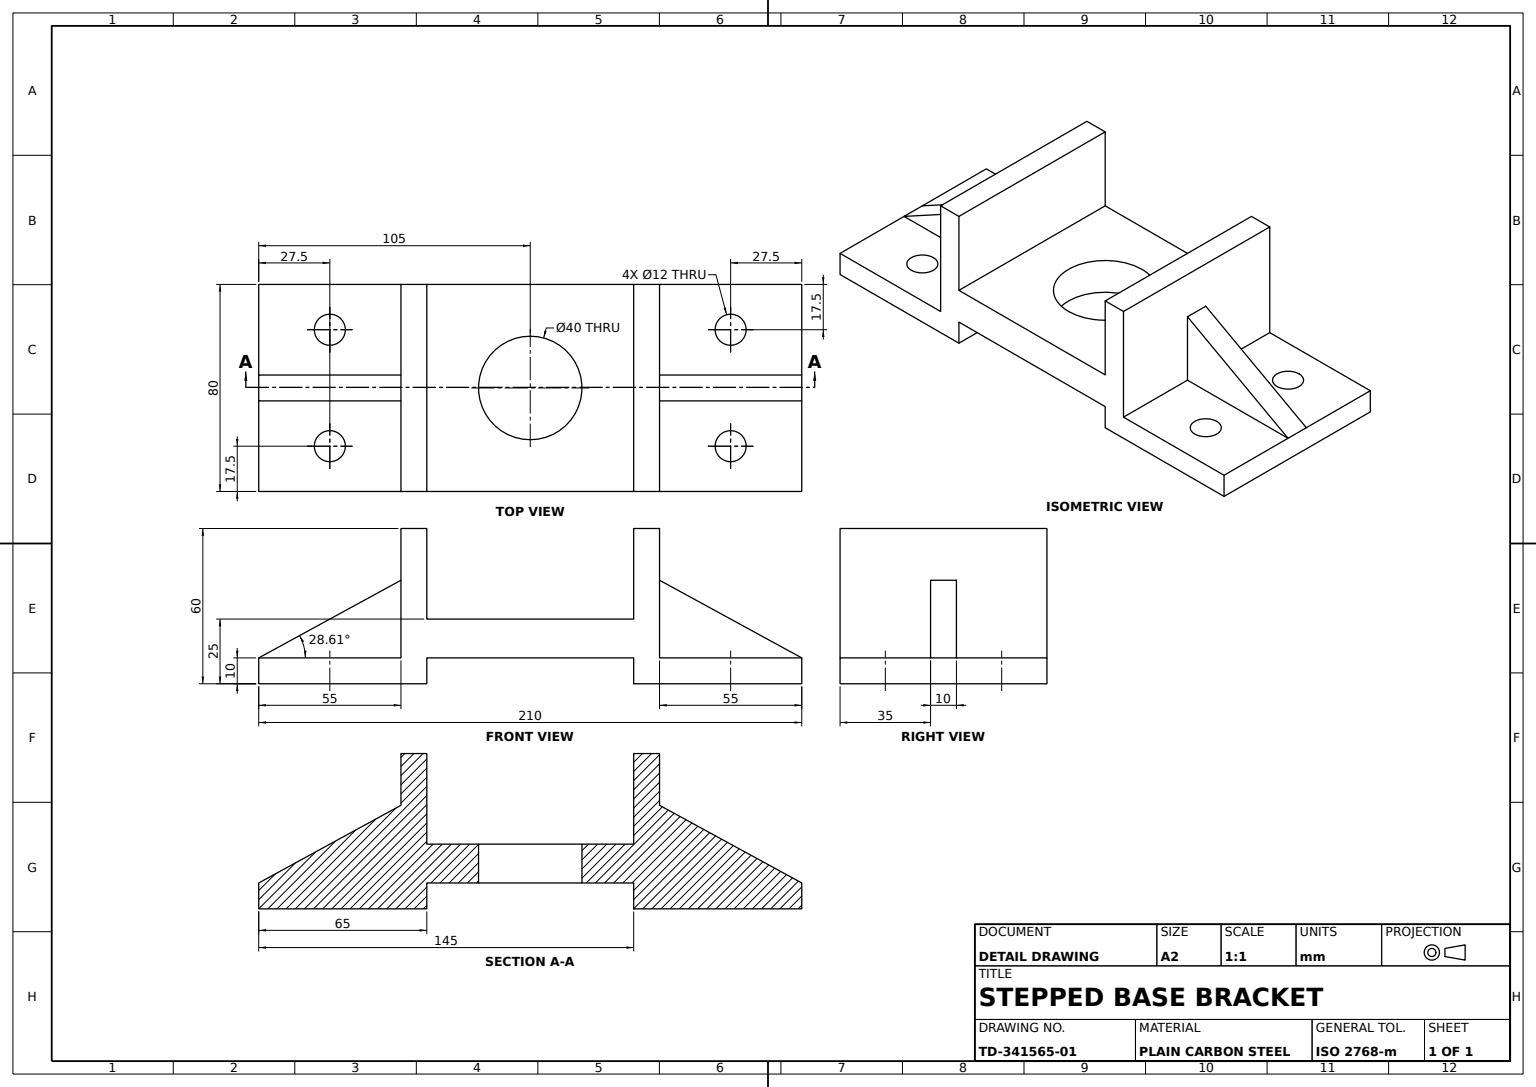
from build123d import *

# Parameters (mm, degrees)
BASE_BODY_DEPTH          = 60
CENTER_BORE_SKETCH_R     = 20
CENTER_BORE_DEPTH        = 15
GUSSET_1_BLANK_DEPTH     = 40
GUSSET_1_TRIM_A_DEPTH    = 25
GUSSET_1_TRIM_B_DEPTH    = 5
GUSSET_2_BLANK_DEPTH     = 35
GUSSET_2_TRIM_DEPTH      = 25
FLANGE_EXTENSION_1_DEPTH = 10
FLANGE_EXTENSION_2_DEPTH = 10
MOUNTING_HOLES_SKETCH_R  = 6
MOUNTING_HOLES_4X_DEPTH  = 10


with BuildPart() as part:
    # Base Profile Sketch → Base Body (new body)
    with BuildSketch(Plane.XY):
        Polygon((0, 0), (55, 0), (65, 0), (65, 10), (145, 10), (145, 0), (210, 0), (210, 10), (155, 10), (155, 60), (145, 60), (145, 25), (65, 25), (65, 60), (55, 60), (55, 10), (0, 10), align=None)
    extrude(amount=BASE_BODY_DEPTH)

    # Center Bore Sketch → Center Bore (cut)
    with BuildSketch(Plane(origin=(0, 25, 0), x_dir=(1, 0, 0), z_dir=(0, 1, 0))):
        with Locations(Location((105, -30, 0), (0, 0, 270))):
            Circle(CENTER_BORE_SKETCH_R)
    extrude(amount=-CENTER_BORE_DEPTH, mode=Mode.SUBTRACT)

    # Gusset 1 Sketch → Gusset 1 Blank (add)
    with BuildSketch(Plane.XY.offset(60)):
        Polygon((155, 10), (155, 40), (210, 10), align=None)
    extrude(amount=-GUSSET_1_BLANK_DEPTH)

    # Gusset 1 Trim A Sketch → Gusset 1 Trim A (cut)
    with BuildSketch(Plane.XY.offset(60)):
        Polygon((155, 40), (155, 10), (210, 10), align=None)
    extrude(amount=-GUSSET_1_TRIM_A_DEPTH, mode=Mode.SUBTRACT)

    # Gusset 1 Trim B Sketch → Gusset 1 Trim B (cut)
    with BuildSketch(Plane(origin=(0, 0, 20), x_dir=(-1, 0, 0), z_dir=(0, 0, -1))):
        Polygon((-210, 10), (-155, 10), (-155, 40), align=None)
    extrude(amount=-GUSSET_1_TRIM_B_DEPTH, mode=Mode.SUBTRACT)

    # Gusset 2 Sketch → Gusset 2 Blank (add)
    with BuildSketch(Plane(origin=(0, 0, 0), x_dir=(-1, 0, 0), z_dir=(0, 0, -1))):
        Polygon((-55, 10), (-55, 40), (0, 10), align=None)
    extrude(amount=-GUSSET_2_BLANK_DEPTH)

    # Gusset 2 Trim Sketch → Gusset 2 Trim (cut)
    with BuildSketch(Plane(origin=(0, 0, 0), x_dir=(-1, 0, 0), z_dir=(0, 0, -1))):
        Polygon((-55, 40), (-55, 10), (0, 10), align=None)
    extrude(amount=-GUSSET_2_TRIM_DEPTH, mode=Mode.SUBTRACT)

    # Flange Extension 1 Sketch → Flange Extension 1 (add)
    with BuildSketch(Plane.XY.offset(60)):
        Polygon((0, 0), (0, 10), (55, 10), (55, 60), (65, 60), (65, 25), (145, 25), (145, 60), (155, 60), (155, 10), (210, 10), (210, 0), (145, 0), (145, 10), (65, 10), (65, 0), align=None)
    extrude(amount=FLANGE_EXTENSION_1_DEPTH)

    # Flange Extension 2 Sketch → Flange Extension 2 (add)
    with BuildSketch(Plane(origin=(0, 0, 0), x_dir=(-1, 0, 0), z_dir=(0, 0, -1))):
        Polygon((-210, 0), (-210, 10), (-155, 10), (-155, 60), (-145, 60), (-145, 25), (-65, 25), (-65, 60), (-55, 60), (-55, 10), (0, 10), (0, 0), (-65, 0), (-65, 10), (-145, 10), (-145, 0), align=None)
    extrude(amount=FLANGE_EXTENSION_2_DEPTH)

    # Mounting Holes Sketch → Mounting Holes 4x (cut)
    with BuildSketch(Plane(origin=(0, 10, 0), x_dir=(1, 0, 0), z_dir=(0, 1, 0))):
        with Locations(Location((27.5, -52.5, 0), (0, 0, 270))):
            Circle(MOUNTING_HOLES_SKETCH_R)
        with Locations(Location((27.5, -7.5, 0), (0, 0, 270))):
            Circle(MOUNTING_HOLES_SKETCH_R)
        with Locations(Location((182.5, -7.5, 0), (0, 0, 270))):
            Circle(MOUNTING_HOLES_SKETCH_R)
        with Locations(Location((182.5, -52.5, 0), (0, 0, 270))):
            Circle(MOUNTING_HOLES_SKETCH_R)
    extrude(amount=-MOUNTING_HOLES_4X_DEPTH, mode=Mode.SUBTRACT)


solid = part.part
